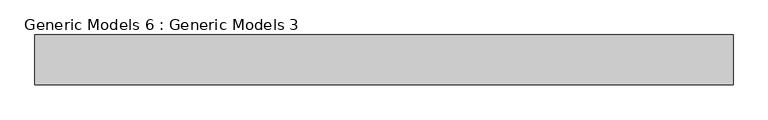
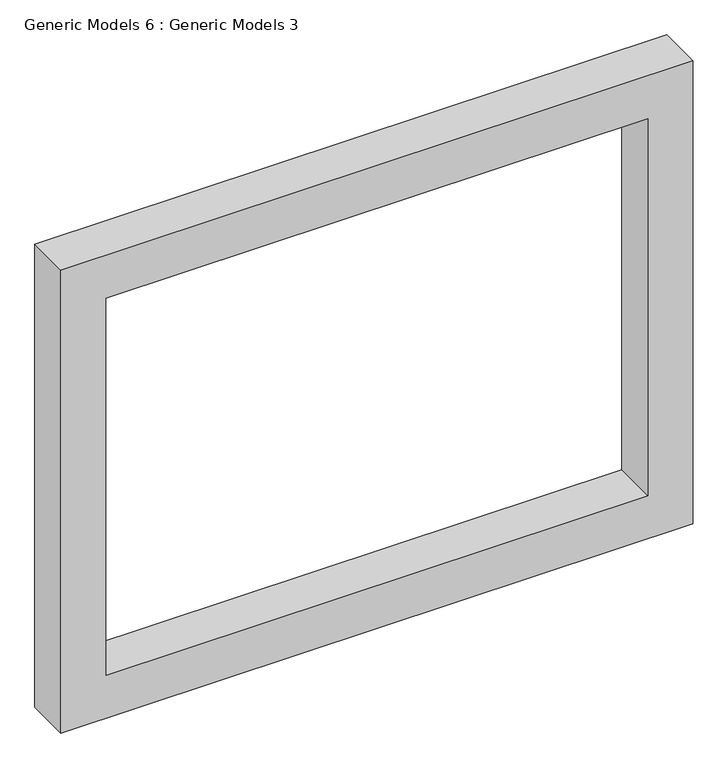
"""IFC4 building model written with IfcOpenShell, lengths in millimetres: proxy geometry, Generic Models 6 : Generic Models 3."""

from ifc_helpers import new_model, si_unit, frame, origin, place, context, project, spatial, polyline, outline, extrude, source, transform, mapped, element, save


def generic_models_6_generic_models_3_5dde034f(model_context):
    return source(origin(), model_context, "Body", "SweptSolid", [
        extrude(outline(polyline([(2717.8, 4569.9671209), (2717.8, 2436.3671209), (1066.8, 2436.3671209), (1066.8, 4569.9671209), (2717.8, 4569.9671209)]), holes=[polyline([(2565.4, 4417.5671209), (1219.2, 4417.5671209), (1219.2, 2588.7671209), (2565.4, 2588.7671209), (2565.4, 4417.5671209)])]), frame((0.0, -2602.2776789, 0.0), z_axis=(0.0, 1.0, 0.0), x_axis=(0.0, 0.0, 1.0)), (0.0, 0.0, 1.0), 152.4),
    ])


if __name__ == "__main__":
    model = new_model("IFC4")
    model_context = context("Model", 3, world=origin())
    ifc_project = project(units=[si_unit("LENGTHUNIT", "METRE", prefix="MILLI")], contexts=[model_context])
    site = spatial("IfcSite", under=ifc_project)
    building = spatial("IfcBuilding", under=site)
    placement = place(None, origin())
    generic_models_6_generic_models_3_shape = generic_models_6_generic_models_3_5dde034f(model_context)
    element("IfcBuildingElementProxy", 1, Name="Generic Models 6 : Generic Models 3", ObjectType="Generic Models 6 : Generic Models 3", at=placement, inside=building, context=model_context, shape_type="MappedRepresentation", body=[
        mapped(generic_models_6_generic_models_3_shape, transform((0.0, 0.0, 0.0), x_axis=(1.0, 0.0, 0.0), y_axis=(0.0, 1.0, 0.0), z_axis=(0.0, 0.0, 1.0))),
    ])
    save(model, "model.ifc")

# Revit data of these elements
# Element 1 (IfcBuildingElementProxy, "Generic Models 6 : Generic Models 3")
#   Materials on its faces: "WALNUT WOOD COLOUR 5\""
# Materials
#   "WALNUT WOOD COLOUR 5\"": class "Generic", colour RGB 120 120 120, transparency 0, Cost = 0
